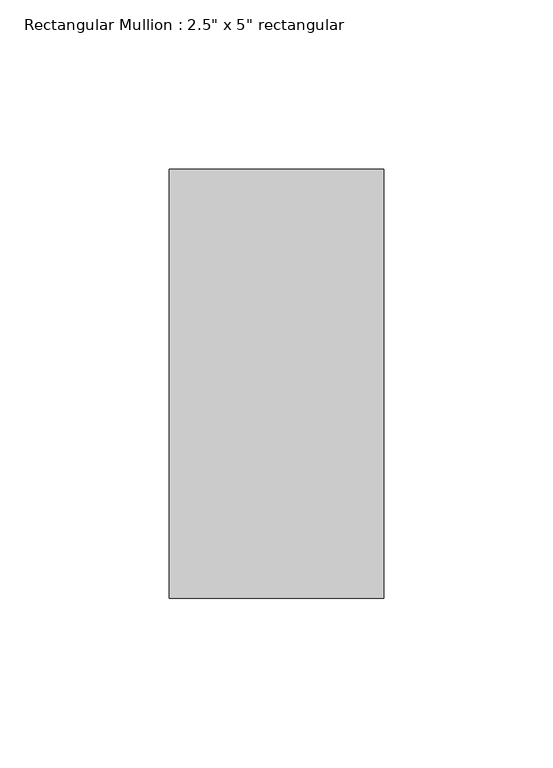
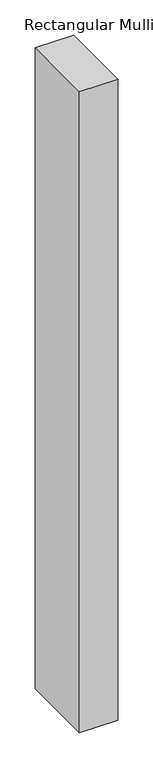
"""IFC4 building model written with IfcOpenShell, lengths in millimetres: member geometry."""

from ifc_helpers import new_model, si_unit, frame, origin, place, context, project, spatial, polyline, outline, extrude, source, transform, mapped, element, save


def member_c95c5e6c(model_context):
    return source(origin(), model_context, "Body", "SweptSolid", [
        extrude(outline(polyline([(31.75, 63.5), (31.75, -63.5), (-31.75, -63.5), (-31.75, 63.5), (31.75, 63.5)])), frame((0.0, 0.0, -1117.5999998), z_axis=(0.0, 0.0, 1.0), x_axis=(1.0, 0.0, 0.0)), (0.0, 0.0, 1.0), 1117.5999998),
    ])


if __name__ == "__main__":
    model = new_model("IFC4")
    model_context = context("Model", 3, world=origin())
    ifc_project = project(units=[si_unit("LENGTHUNIT", "METRE", prefix="MILLI")], contexts=[model_context])
    site = spatial("IfcSite", under=ifc_project)
    building = spatial("IfcBuilding", under=site)
    placement = place(None, origin())
    member_shape = member_c95c5e6c(model_context)
    element("IfcMember", 1, ObjectType="Rectangular Mullion : 2.5\" x 5\" rectangular", at=placement, inside=building, context=model_context, shape_type="MappedRepresentation", body=[
        mapped(member_shape, transform((0.0, 0.0, 0.0), x_axis=(1.0, 0.0, 0.0), y_axis=(0.0, 1.0, 0.0), z_axis=(0.0, 0.0, 1.0))),
    ])
    save(model, "model.ifc")

# Revit data of these elements
# Type "Rectangular Mullion : 2.5\" x 5\" rectangular"
#   built-in parameter 1007304 = 0.416667 (stored number, unit not read)
#   built-in parameter 1007301 = 0.104167 (stored number, unit not read)
#   built-in parameter 1007300 = 0.104167 (stored number, unit not read)
# Element 1 (IfcMember, "Rectangular Mullion : 2.5\" x 5\" rectangular")
#   Materials on its faces: "Aluminum"
# Materials
#   "Aluminum": class "Metal", colour RGB 247 247 247, transparency 0, Description = "Aluminum 6061", Cost = 0
